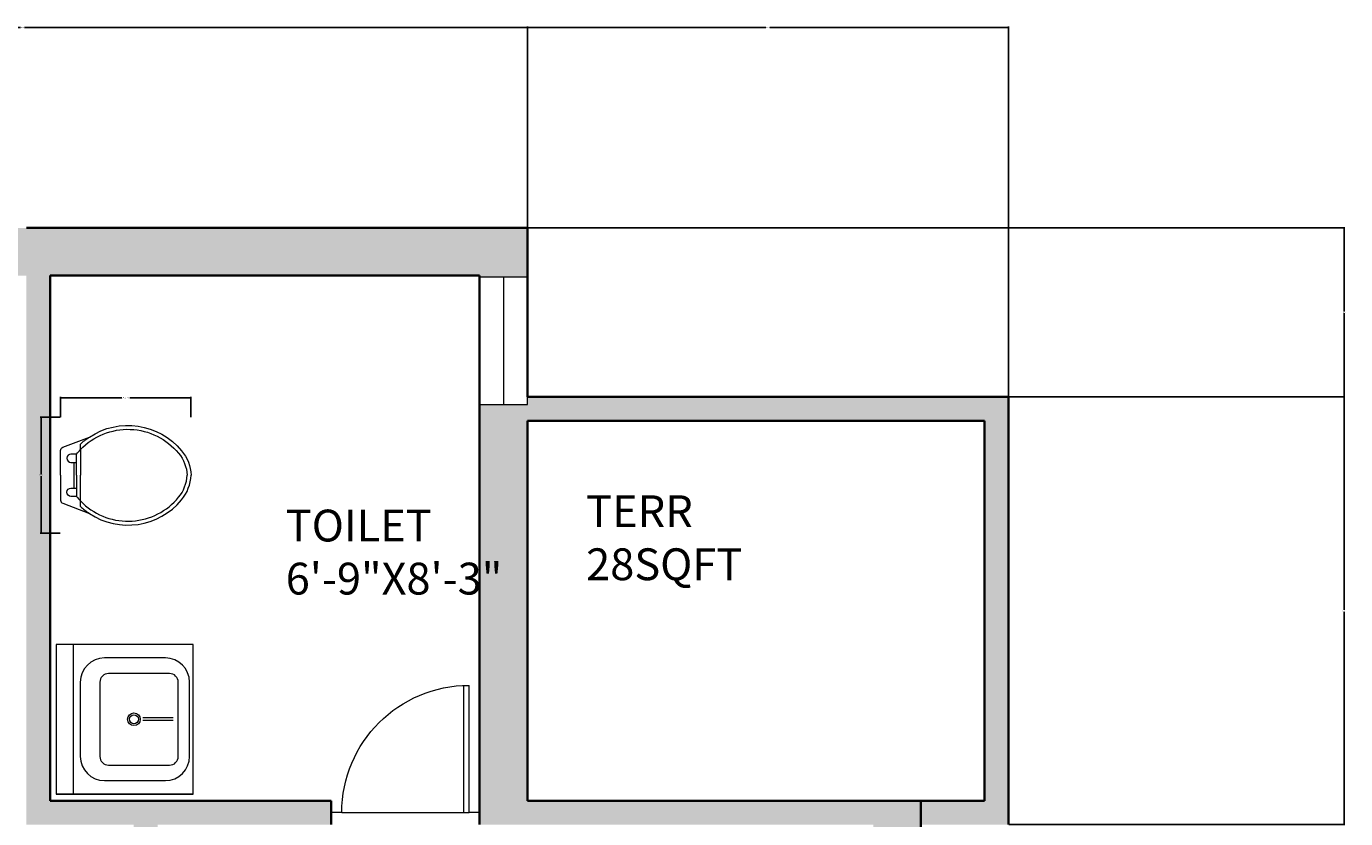
# Model space of a CAD drawing. Units: inches. Extents: x -36 to 442, y -676 to 151.
# Tile 8 of 8: x 193 to 442, y 2 to 151. Entities that reach past the tile are written whole.
import ezdxf

# ---------------------------------------------------------------- set-up
doc = ezdxf.new("R2010")
doc.units = ezdxf.units.IN
doc.header["$MEASUREMENT"] = 0
for name, color, linetype, lineweight in [('A-ANNO-DIMS', 2, 'Continuous', 18), ('A-AREA-IDEN', 7, 'Continuous', 18), ('A-DOOR', 4, 'Continuous', 18), ('A-FLOR-FIXT', 9, 'Continuous', 18), ('A-GLAZ', 4, 'Continuous', 13), ('A-WALL', 7, 'Continuous', 35), ('A-WALL-PATT', 8, 'Continuous', 13)]:
    doc.layers.add(name, color=color, linetype=linetype, lineweight=lineweight)
doc.styles.get("Standard").update_dxf_attribs({"font": 'arial.ttf'})
doc.dimstyles.get("Standard").update_dxf_attribs({"dimtxt": 0.18, "dimasz": 0.18, "dimexe": 0.18, "dimexo": 0.0625, "dimgap": 0.09, "dimtad": 0, "dimtih": 1, "dimtoh": 1, "dimdec": 0, "dimzin": 0, "dimdsep": 46, "dimlunit": 3, "dimtxsty": 'Standard', "dimcen": 0.09, "dimadec": 0, "dimazin": 0, "dimtfac": 1, "dimtdec": 0, "dimtofl": 0, "dimtmove": 0, "dimatfit": 3, "dimfxl": 1, "dimtolj": 1, "dimtzin": 0, "dimarcsym": 0})

# ---------------------------------------------------------------- blocks, each defined once
blk = doc.blocks.new('М14 600х655')
for p, q in [((-655, 600), (-655, 0)), ((-655, 600), (-655, 0)), ((-655, 0), (-655, 600)), ((0, 600), (-655, 600)), ((0, 0), (0, 600)), ((0, 525), (-655, 525)), ((-165.1, 494.1), (-489.9, 494.1)), ((-165.4, 408.4), (-490.2, 408.4)), ((-595.8, 388.1), (-595.8, 121.3)), ((-528.4, 370.1), (-528.4, 103.3)), ((-127.2, 103.3), (-127.2, 370.1)), ((-59.2, 121.3), (-59.2, 388.1)), ((-333.5, 87.1), (-333.5, 219.6)), ((-321.5, 87.1), (-321.5, 219.6)), ((-490.2, 65.1), (-165.4, 65.1)), ((-655, 0), (-655, 0)), ((-655, 0), (-655, 0)), ((-655, 0), (0, 0)), ((-655, 0), (0, 0)), ((-489.9, 15.4), (-165.1, 15.4))]:
    blk.add_line(p, q)
for radius in [27.6, 19.3]:
    blk.add_circle((-327.5, 258.9), radius)
for centre, radius, start, end in [((-489.9, 388.1), 105.9, 90, 180), ((-165.1, 388.1), 105.9, 0, 90), ((-490.2, 370.1), 38.2, 90, 180), ((-165.4, 370.1), 38.2, 0, 90), ((-489.9, 121.3), 105.9, 180, 270), ((-165.1, 121.3), 105.9, 270, 0), ((-490.2, 103.3), 38.2, 180, 270), ((-165.4, 103.3), 38.2, 270, 0)]:
    blk.add_arc(centre, radius, start, end)
blk = doc.blocks.new('DOOR-SWING-24IN')
for p, q in [((24, 26), (24, 28)), ((24, 26), (24, 2)), ((24, 3), (0, 3)), ((24, 2), (0, 2)), ((24, 0), (24, 2))]:
    blk.add_line(p, q)
blk.add_arc((24, 2), 24, 90, 180)
blk = doc.blocks.new('WC-PLAN')
for p, q in [((3.72, 14.23), (3.72, 15.26)), ((3.72, 14.23), (3.72, 9.39)), ((3.72, 4.56), (3.72, 9.39)), ((3.72, 3.52), (3.72, 4.56))]:
    blk.add_line(p, q)
for points in [[(3.72, 14.23, -0.448546), (22.25, 13.55, -0.162618), (23.85, 9.39, -0.470877)], [(5.41, 16.59, -0.383919), (22.82, 14.02, -0.163732), (24.59, 9.39, -0.359733)], [(0, 9.39), (0, 14.09, -0.31031), (0.4, 14.66), (5.41, 16.59, -0.209071)], [(3.72, 15.26, -0.040937), (5.41, 16.59, -0.163732)], [(2.98, 13.38), (1.95, 13.38, 1), (1.95, 11.81), (2.49, 11.81)], [(2.98, 13.38, -0.022712), (3.72, 14.23, -0.162618)], [(2.98, 9.39), (2.98, 13.38, -0.476108)], [(0, 9.39), (0, 4.7, 0.31031), (0.4, 4.12), (5.41, 2.19, 0.209071)], [(2.98, 9.39), (2.98, 5.4, 0.022712)], [(4.22, 4.06, 0.431639), (22.25, 5.24, 0.162618), (23.85, 9.39, 0.470877)], [(5.41, 2.19, 0.383919), (22.82, 4.77, 0.163732), (24.59, 9.39, 0.359733)], [(2.98, 5.4), (1.95, 5.4, -1), (1.95, 6.97), (2.49, 6.97)], [(2.98, 5.4, 0.022712), (3.72, 4.56, 0.162618)], [(3.72, 4.56, 0.014165), (4.22, 4.06, 0.162618)], [(3.72, 3.52, 0.040937), (5.41, 2.19, 0.163732)]]:
    blk.add_lwpolyline(points, format="xyb")
for points in [[(2.49, 11.81), (2.49, 6.97)], [(2.49, 11.81), (2.98, 11.81)], [(2.49, 6.97), (2.98, 6.97)]]:
    blk.add_lwpolyline(points)
blk = doc.blocks.new('*D29')
at = {"layer": 'A-ANNO-DIMS', "color": 0, "lineweight": -2, "transparency": 16777216}
for p, q in [((199.96, 77.84), (199.96, 81.65)), ((200.14, 81.47), (211.48, 81.47)), ((224.37, 81.47), (213.03, 81.47)), ((224.55, 77.84), (224.55, 81.65))]:
    blk.add_line(p, q, dxfattribs=at)
at = {"layer": 'A-ANNO-DIMS', "color": 0, "transparency": 16777216}
for points in [[(200.14, 81.5), (200.14, 81.44), (199.96, 81.47)], [(224.37, 81.5), (224.37, 81.44), (224.55, 81.47)]]:
    blk.add_solid(points, dxfattribs=at)
at = {"layer": 'Defpoints', "color": 0, "transparency": 16777216}
for p in [(224.55, 81.47), (199.96, 77.78), (224.55, 77.78)]:
    blk.add_point(p, dxfattribs=at)
at = {"layer": 'A-ANNO-DIMS', "color": 0, "transparency": 16777216, "insert": (212.26, 81.47), "char_height": 0.18, "attachment_point": 5}
blk.add_mtext('\\A1;WC 25 TYP.', dxfattribs=at)
blk = doc.blocks.new('*D30')
at = {"layer": 'A-ANNO-DIMS', "color": 0, "lineweight": -2, "transparency": 16777216}
for p, q in [((199.9, 77.78), (196.1, 77.78)), ((196.28, 77.6), (196.28, 67.04)), ((196.28, 56.12), (196.28, 66.68)), ((199.9, 55.94), (196.1, 55.94))]:
    blk.add_line(p, q, dxfattribs=at)
at = {"layer": 'A-ANNO-DIMS', "color": 0, "transparency": 16777216}
for points in [[(196.25, 77.6), (196.31, 77.6), (196.28, 77.78)], [(196.25, 56.12), (196.31, 56.12), (196.28, 55.94)]]:
    blk.add_solid(points, dxfattribs=at)
at = {"layer": 'Defpoints', "color": 0, "transparency": 16777216}
for p in [(196.28, 77.78), (199.96, 77.78), (199.96, 55.94)]:
    blk.add_point(p, dxfattribs=at)
at = {"layer": 'A-ANNO-DIMS', "color": 0, "transparency": 16777216, "insert": (196.28, 66.86), "char_height": 0.18, "attachment_point": 5}
blk.add_mtext('\\A1;22 TYP.', dxfattribs=at)
blk = doc.blocks.new('*D52')
at = {"layer": 'A-ANNO-DIMS', "color": 0, "lineweight": -2, "transparency": 16777216}
for p, q in [((97.5, 113.57), (97.5, 151.48)), ((97.68, 151.3), (192.36, 151.3)), ((287.82, 151.3), (193.14, 151.3)), ((288, 113.57), (288, 151.48))]:
    blk.add_line(p, q, dxfattribs=at)
at = {"layer": 'A-ANNO-DIMS', "color": 0, "transparency": 16777216}
for points in [[(97.68, 151.33), (97.68, 151.27), (97.5, 151.3)], [(287.82, 151.33), (287.82, 151.27), (288, 151.3)]]:
    blk.add_solid(points, dxfattribs=at)
at = {"layer": 'Defpoints', "color": 0, "transparency": 16777216}
for p in [(288, 151.3), (97.5, 113.5), (288, 113.5)]:
    blk.add_point(p, dxfattribs=at)
at = {"layer": 'A-ANNO-DIMS', "color": 0, "transparency": 16777216, "insert": (192.75, 151.3), "char_height": 0.18, "attachment_point": 5}
blk.add_mtext('\\A1;190.5', dxfattribs=at)
blk = doc.blocks.new('*D53')
at = {"layer": 'A-ANNO-DIMS', "color": 0, "lineweight": -2, "transparency": 16777216}
for p, q in [((288, 113.57), (288, 151.48)), ((288.18, 151.3), (332.97, 151.3)), ((378.56, 151.3), (333.76, 151.3)), ((378.74, 81.71), (378.74, 151.48))]:
    blk.add_line(p, q, dxfattribs=at)
at = {"layer": 'A-ANNO-DIMS', "color": 0, "transparency": 16777216}
for points in [[(288.18, 151.33), (288.18, 151.27), (288, 151.3)], [(378.56, 151.33), (378.56, 151.27), (378.74, 151.3)]]:
    blk.add_solid(points, dxfattribs=at)
at = {"layer": 'Defpoints', "color": 0, "transparency": 16777216}
for p in [(378.74, 151.3), (288, 113.5), (378.74, 81.65)]:
    blk.add_point(p, dxfattribs=at)
at = {"layer": 'A-ANNO-DIMS', "color": 0, "transparency": 16777216, "insert": (333.37, 151.3), "char_height": 0.18, "attachment_point": 5}
blk.add_mtext('\\A1;90.74', dxfattribs=at)
blk = doc.blocks.new('*D55')
at = {"layer": 'A-ANNO-DIMS', "color": 0, "lineweight": -2, "transparency": 16777216}
for p, q in [((288.06, 113.5), (442.22, 113.5)), ((442.04, 113.32), (442.04, 97.76)), ((442.04, 81.83), (442.04, 97.39)), ((378.8, 81.65), (442.22, 81.65))]:
    blk.add_line(p, q, dxfattribs=at)
at = {"layer": 'A-ANNO-DIMS', "color": 0, "transparency": 16777216}
for points in [[(442.01, 113.32), (442.07, 113.32), (442.04, 113.5)], [(442.01, 81.83), (442.07, 81.83), (442.04, 81.65)]]:
    blk.add_solid(points, dxfattribs=at)
at = {"layer": 'Defpoints', "color": 0, "transparency": 16777216}
for p in [(288, 113.5), (378.74, 81.65), (442.04, 81.65)]:
    blk.add_point(p, dxfattribs=at)
at = {"layer": 'A-ANNO-DIMS', "color": 0, "transparency": 16777216, "insert": (442.04, 97.57), "char_height": 0.18, "attachment_point": 5}
blk.add_mtext('\\A1;31.86', dxfattribs=at)
blk = doc.blocks.new('*D56')
at = {"layer": 'A-ANNO-DIMS', "color": 0, "lineweight": -2, "transparency": 16777216}
for p, q in [((378.8, 81.65), (442.22, 81.65)), ((442.04, 81.47), (442.04, 41.51)), ((442.04, 1.18), (442.04, 41.14)), ((378.8, 1), (442.22, 1))]:
    blk.add_line(p, q, dxfattribs=at)
at = {"layer": 'A-ANNO-DIMS', "color": 0, "transparency": 16777216}
for points in [[(442.01, 81.47), (442.07, 81.47), (442.04, 81.65)], [(442.01, 1.18), (442.07, 1.18), (442.04, 1)]]:
    blk.add_solid(points, dxfattribs=at)
at = {"layer": 'Defpoints', "color": 0, "transparency": 16777216}
for p in [(378.74, 81.65), (378.74, 1), (442.04, 1)]:
    blk.add_point(p, dxfattribs=at)
at = {"layer": 'A-ANNO-DIMS', "color": 0, "transparency": 16777216, "insert": (442.04, 41.32), "char_height": 0.18, "attachment_point": 5}
blk.add_mtext('\\A1;80.64', dxfattribs=at)

msp = doc.modelspace()

# ---------------------------------------------------------------- hatches: boundary and pattern name
at = {"layer": 'A-WALL-PATT'}
h = msp.add_hatch(color=256, dxfattribs=at)
h.dxf.hatch_style = 1
h.paths.add_polyline_path([(288, 113.503), (193.5, 113.503), (97.5, 113.503), (97.5, 104.864), (106.5, 104.864), (106.5, 104.503), (193.5, 104.503), (193.5, 5.503), (193.5, 1.003), (213.735, 1.003), (213.735, -135.497), (218.235, -135.497), (218.235, 1.003), (251, 1.003), (251, 3.253), (251, 5.503), (198, 5.503), (198, 104.503), (279, 104.503), (279, 104.209), (288, 104.209)])
h.paths.add_polyline_path([(378.735, 81.646), (362.235, 81.646), (288, 81.646), (288, 80.209), (279, 80.209), (279, 5.503), (279, 1.003), (353.235, 1.003), (353.235, 0.242), (362.235, 0.242), (362.235, 5.503), (288, 5.503), (288, 77.146), (362.235, 77.146), (374.235, 77.146), (374.235, 5.503), (362.235, 5.503), (362.235, 1.003), (374.235, 1.003), (378.735, 1.003), (378.735, 5.503), (378.735, 77.146)])
h.paths.add_polyline_path([(362.235, -35.758), (353.235, -35.758), (353.235, -196.997), (218.235, -196.997), (213.735, -196.997), (213.735, -205.997), (218.235, -205.997), (378.735, -205.997), (378.735, -205.779), (387.735, -205.779), (387.735, -202.472), (387.735, -196.997), (378.735, -196.997), (362.235, -196.997)])
h.paths.add_polyline_path([(218.235, -175.497), (215.985, -175.497), (213.735, -175.497), (213.735, -196.997), (218.235, -196.997)], flags=17)
h.paths.add_polyline_path([(158.235, -201.497), (98.235, -201.497), (98.235, -205.997), (158.235, -205.997)])
h.paths.add_polyline_path([(173.735, -130.997), (27.735, -130.997), (27.735, -35.267), (18.735, -35.267), (18.735, -138.68), (27.735, -138.68), (27.735, -135.497), (93.735, -135.497), (93.735, -201.497), (98.235, -201.497), (98.235, -135.497), (158.235, -135.497), (158.235, -173.497), (160.739, -173.497), (162.735, -173.497), (162.735, -135.497), (173.735, -135.497), (173.735, -133.017)])
h.paths.add_polyline_path([(98.235, -201.497), (93.735, -201.497), (93.735, -205.997), (98.235, -205.997)])
h.paths.add_polyline_path([(162.735, -201.497), (158.235, -201.497), (158.235, -205.997), (162.735, -205.997)])
h.paths.add_polyline_path([(63.735, -205.997), (63.735, -201.497), (27.735, -201.497), (27.735, -162.68), (18.735, -162.68), (18.735, -210.497), (63.735, -210.497)])
h.paths.add_polyline_path([(65.735, -203.604), (65.735, -201.497), (63.735, -201.497), (63.735, -205.997), (65.735, -205.997)])
h.paths.add_polyline_path([(165.5, 5.503), (106.5, 5.503), (106.5, 80.864), (97.5, 80.864), (97.5, 81.646), (6.735, 81.646), (2.235, 81.646), (2.235, 77.146), (2.235, 5.503), (2.235, 1.003), (6.735, 1.003), (18.735, 1.003), (18.735, 5.503), (6.735, 5.503), (6.735, 77.146), (97.5, 77.146), (97.5, 5.503), (18.735, 5.503), (18.735, 0.733), (27.735, 0.733), (27.735, 1.003), (165.5, 1.003), (165.5, 3.253)])
h.paths.add_polyline_path([(18.735, -201.497), (6.735, -201.497), (2.235, -201.497), (2.235, -210.497), (2.235, -354.497), (2.235, -363.497), (6.735, -363.497), (18.735, -363.497), (18.735, -358.997), (18.735, -354.497), (6.735, -354.497), (6.735, -210.497), (18.735, -210.497)])
h.paths.add_polyline_path([(63.735, -210.497), (54.735, -210.497), (54.735, -240.747), (63.735, -240.747)])
h.paths.add_polyline_path([(63.735, -336.747), (54.735, -336.747), (54.735, -354.497), (18.735, -354.497), (18.735, -358.997), (18.735, -363.497), (104.735, -363.497), (104.735, -361.247), (104.735, -358.997), (63.735, -358.997)])
h.paths.add_polyline_path([(27.735, -448.151), (18.735, -448.151), (18.735, -637.997), (72.735, -637.997), (72.735, -571.997), (183.235, -571.997), (183.235, -562.997), (57.197, -562.997), (51.735, -562.997), (51.735, -567.497), (57.197, -567.497), (63.735, -567.497), (63.735, -571.997), (63.735, -628.997), (27.735, -628.997), (27.735, -475.997), (27.735, -471.497)])
h.paths.add_polyline_path([(27.735, -363.497), (18.735, -363.497), (18.735, -412.151), (27.735, -412.151)])
h.paths.add_polyline_path([(161.235, -358.997), (132.735, -358.997), (132.735, -363.497), (156.735, -363.497), (156.735, -471.497), (51.735, -471.497), (51.735, -475.997), (63.735, -475.997), (63.735, -534.997), (65.985, -534.997), (68.235, -534.997), (68.235, -475.997), (161.235, -475.997)])
h.paths.add_polyline_path([(161.235, -511.997), (173.235, -511.997), (173.235, -502.997), (161.235, -502.997), (161.235, -475.997), (152.235, -475.997), (152.235, -534.997), (156.735, -534.997), (161.235, -534.997)], flags=17)
h.paths.add_polyline_path([(362.235, -502.997), (353.235, -502.997), (213.235, -502.997), (213.235, -507.497), (213.235, -511.997), (362.235, -511.997)])
h.paths.add_polyline_path([(242.235, -548.019), (233.235, -548.019), (233.235, -562.997), (223.235, -562.997), (223.235, -567.497), (223.235, -571.997), (242.235, -571.997)])
h.paths.add_polyline_path([(404.235, -502.997), (399.735, -502.997), (362.235, -502.997), (362.235, -511.997), (399.735, -511.997), (404.235, -511.997)])
h.paths.add_polyline_path([(362.235, -482.123), (353.235, -482.123), (353.235, -502.997), (362.235, -502.997)])
h.paths.add_polyline_path([(404.235, -295.997), (404.235, -286.997), (387.735, -286.997), (387.735, -295.997), (399.735, -295.997), (399.735, -502.997), (404.235, -502.997)])
h.paths.add_polyline_path([(362.235, -355.863), (353.235, -355.863), (353.235, -386.123), (362.235, -386.123)])
h.paths.add_polyline_path([(387.735, -286.997), (378.735, -286.997), (213.735, -286.997), (213.735, -295.997), (353.235, -295.997), (353.235, -295.863), (362.235, -295.863), (362.235, -295.997), (378.735, -295.997), (387.735, -295.997)])
h.paths.add_polyline_path([(387.735, -241.779), (378.735, -241.779), (378.735, -286.997), (387.735, -286.997)])
h.paths.add_polyline_path([(387.735, -175.497), (362.235, -175.497), (362.235, -184.497), (387.735, -184.497)], flags=17)
h.paths.add_polyline_path([(387.735, -184.497), (383.235, -184.497), (383.235, -192.497), (378.735, -192.497), (366.735, -192.497), (366.735, -184.497), (362.235, -184.497), (362.235, -196.997), (378.735, -196.997), (387.735, -196.997)], flags=17)
h.paths.add_polyline_path([(240.604, 40.967), (282.575, 40.967), (282.575, 63.356), (240.604, 63.356)], flags=25)

# ---------------------------------------------------------------- linework, layer by layer
at = {"layer": 'A-GLAZ'}
for p, q in [((279, 104.209), (279, 80.209)), ((288, 104.209), (279, 104.209)), ((283.5, 104.209), (283.5, 80.209)), ((288, 80.209), (288, 104.209)), ((279, 80.209), (288, 80.209))]:
    msp.add_line(p, q, dxfattribs=at)
at = {"layer": 'A-WALL'}
for p, q in [((193.5, 113.503), (288, 113.503)), ((288, 81.646), (288, 113.503)), ((198, 5.503), (198, 104.503)), ((198, 104.503), (279, 104.503)), ((279, 5.503), (279, 104.503)), ((288, 81.646), (362.235, 81.646)), ((362.235, 81.646), (378.735, 81.646)), ((378.735, 81.646), (378.735, 77.146)), ((288, 5.503), (288, 77.146)), ((288, 77.146), (362.235, 77.146)), ((374.235, 77.146), (362.235, 77.146)), ((374.235, 5.503), (374.235, 77.146)), ((378.735, 5.503), (378.735, 77.146)), ((198, 5.503), (251, 5.503)), ((251, 3.253), (251, 5.503)), ((279, 5.503), (279, 1.003)), ((288, 5.503), (362.235, 5.503)), ((362.235, 5.503), (362.235, -196.997)), ((362.235, 5.503), (374.235, 5.503)), ((378.735, 1.003), (378.735, 5.503)), ((251, 3.253), (251, 1.003))]:
    msp.add_line(p, q, dxfattribs=at)

# ---------------------------------------------------------------- block references
at = {"layer": 'A-DOOR', "extrusion": (0, 0, -1), "zscale": -1, "rotation": 270.0000000000004}
msp.add_blockref('DOOR-SWING-24IN', (-279, 27.253), dxfattribs=at)
at = {"layer": 'A-FLOR-FIXT'}
msp.add_blockref('WC-PLAN', (199.964, 57.466), dxfattribs=at)
at = {"layer": 'A-FLOR-FIXT', "xscale": 0.0430748895547816, "yscale": 0.0430748895547816, "zscale": 0.0430748895547816, "rotation": 90}
msp.add_blockref('М14 600х655', (224.94, 34.962), dxfattribs=at)

# ---------------------------------------------------------------- texts
at = {"layer": 'A-AREA-IDEN', "char_height": 6, "attachment_point": 1}
for s, insert in [('TERR\\P28SQFT', (299.083, 63.079)), ('TOILET\\P6\'-9"X8\'-3"', (242.419, 60.375))]:
    msp.add_mtext(s, dxfattribs=dict(at, insert=insert))

# ---------------------------------------------------------------- dimensions: what is measured, and where the dimension line sits
at = {"layer": 'A-ANNO-DIMS'}
for base, p1, p2, override, picture, middle in [((288, 151.303), (97.5, 113.503), (288, 113.503), {"dimdec": 1, "dimlfac": 1, "dimrnd": 0, "dimzin": 0, "dimdsep": 46, "dimlunit": 2}, '*D52', (192.75, 151.303)), ((378.7351, 151.303), (287.9998, 113.503), (378.7351, 81.6458), {"dimdec": 2, "dimlfac": 1, "dimrnd": 0, "dimzin": 0, "dimdsep": 46, "dimlunit": 2}, '*D53', (333.3674, 151.303))]:
    dim = msp.add_linear_dim(base=base, p1=p1, p2=p2, dimstyle='Standard', override=override, dxfattribs=at)
    dim.commit()
    dim.dimension.update_dxf_attribs({"geometry": picture, "text_midpoint": middle})
for base, p1, p2, picture, middle in [((442.035, 81.646), (288, 113.503), (378.735, 81.646), '*D55', (442.035, 97.574)), ((442.035, 1.003), (378.735, 81.646), (378.735, 1.003), '*D56', (442.035, 41.324))]:
    dim = msp.add_linear_dim(base=base, p1=p1, p2=p2, angle=90, dimstyle='Standard', override={"dimdec": 2, "dimlfac": 1, "dimrnd": 0, "dimzin": 0, "dimdsep": 46, "dimlunit": 2}, dxfattribs=at)
    dim.commit()
    dim.dimension.update_dxf_attribs({"geometry": picture, "text_midpoint": middle})
dim = msp.add_linear_dim(base=(224.551, 81.47), p1=(199.964, 77.782), p2=(224.551, 77.782), text='WC <> TYP.', dimstyle='Standard', override={"dimdec": 0, "dimlfac": 1, "dimrnd": 0, "dimzin": 0, "dimdsep": 46, "dimlunit": 2}, dxfattribs=at)
dim.commit()
dim.dimension.update_dxf_attribs({"geometry": '*D29', "text_midpoint": (212.258, 81.47)})
dim = msp.add_linear_dim(base=(196.276, 77.782), p1=(199.964, 55.938), p2=(199.964, 77.782), angle=90, text='<> TYP.', dimstyle='Standard', override={"dimdec": 0, "dimlfac": 1, "dimrnd": 0, "dimzin": 0, "dimdsep": 46, "dimlunit": 2}, dxfattribs=at)
dim.commit()
dim.dimension.update_dxf_attribs({"geometry": '*D30', "text_midpoint": (196.276, 66.86)})

doc.saveas('drawing.dxf')
